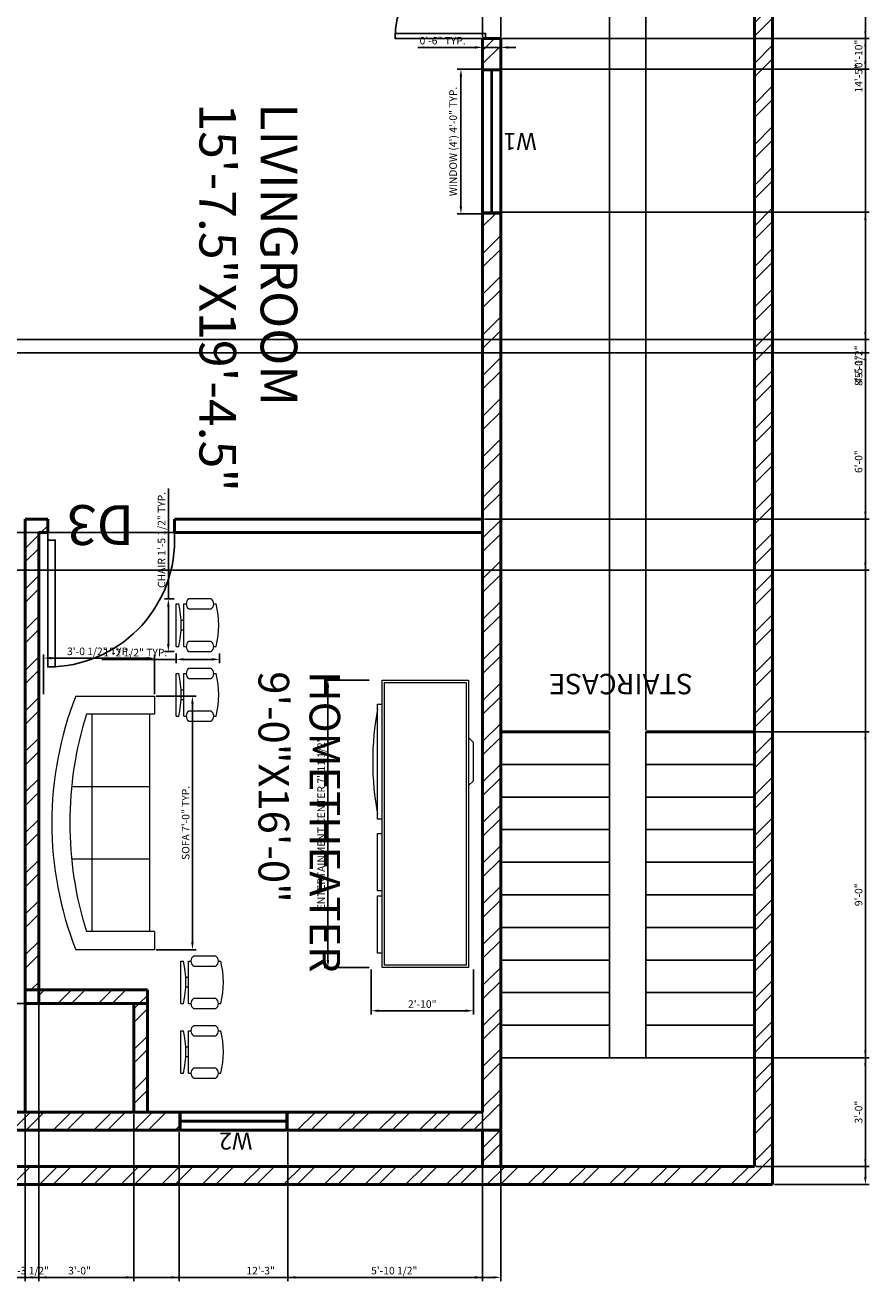
# Model space of a CAD drawing. Units: inches. Extents: x 244 to 2800, y 1060 to 1700.
# Tile 4 of 13: x 1088 to 1368, y 1060 to 1477. Entities that reach past the tile are written whole.
import ezdxf

# ---------------------------------------------------------------- set-up
doc = ezdxf.new("R2010")
doc.units = ezdxf.units.IN
for name, color, linetype, lineweight in [('A-ANNO-DIMS', 2, 'Continuous', 18), ('A-ANNO-TEXT', 1, 'Continuous', 18), ('A-DOOR', 5, 'Continuous', 25), ('A-FLOR-STRS', 6, 'Continuous', 25), ('A-FURN', 9, 'Continuous', 18), ('A-GLAZ', 3, 'Continuous', 25), ('A-WALL', 7, 'Continuous', 50), ('A-WALL-PATT', 8, 'Continuous', 13)]:
    doc.layers.add(name, color=color, linetype=linetype, lineweight=lineweight)
doc.styles.get("Standard").update_dxf_attribs({"font": 'arial.ttf'})
doc.dimstyles.new('ISO-25', dxfattribs={"dimtxt": 2.5, "dimasz": 2.5, "dimexe": 1.25, "dimexo": 0.625, "dimtad": 1, "dimlunit": 4, "dimtxsty": 'Standard', "dimcen": 2.5, "dimadec": 0, "dimazin": 0, "dimtfac": 1, "dimtmove": 0, "dimatfit": 3, "dimfxl": 1, "dimarcsym": 0})

# ---------------------------------------------------------------- blocks, each defined once
blk = doc.blocks.new('*U2')
for p, q in [((0, 0), (0, -5)), ((30, 0), (30, -5))]:
    blk.add_line(p, q)
blk.add_lwpolyline([(0, 0), (0, 30), (1.75, 30), (1.75, 0)], close=True)
blk.add_arc((0, 0), 30, 0, 90)
blk = doc.blocks.new('Entertainment Center')
for p, q in [((-4, 0), (-5, -1)), ((4, 0), (-4, 0)), ((5, -1), (4, 0)), ((-17, -19), (-17, -1)), ((-17, -1), (43, -1)), ((-16.5, -18.5), (-16.5, -1.5)), ((-16.5, -1.5), (42.5, -1.5)), ((42.5, -1.5), (42.5, -18.5)), ((43, -1), (43, -19)), ((43, -19), (-17, -19)), ((42.5, -18.5), (-16.5, -18.5)), ((-12, -20), (-12, -19)), ((12, -20), (-12, -20)), ((12, -19), (12, -20)), ((15, -20), (15, -19)), ((27, -20), (15, -20)), ((27, -19), (27, -20)), ((28, -20), (28, -19)), ((40, -20), (28, -20)), ((40, -19), (40, -20))]:
    blk.add_line(p, q)
blk.add_arc((0, 40), 61, 259.6111, 280.3889)
blk = doc.blocks.new('Chair - Desk')
for p, q in [((-8.5, 0), (-8.5, -1)), ((-8.5, 0), (8.5, 0)), ((8.5, 0), (8.5, -1)), ((-10.5, -5), (-10.5, -14)), ((-8.5, -3), (-8.5, -4)), ((-8.5, -3), (8.5, -3)), ((-6.5, -14), (-6.5, -5)), ((-2, -3), (-2, -1.9355)), ((2, -1.9576), (2, -3)), ((6.5, -5), (6.5, -14)), ((8.5, -3), (8.5, -4)), ((10.5, -14), (10.5, -5)), ((-8.5, -15), (-8.5, -16)), ((8.5, -15), (8.5, -16))]:
    blk.add_line(p, q)
for centre, radius, start, end in [((-8.5, -6.5), 2.5, 36.8699, 143.1301), ((0, 34.625), 36.625, 256.5803, 283.4197), ((8.5, -6.5), 2.5, 36.8699, 143.1301), ((-8.5, -12.5), 2.5, 216.8699, 323.1301), ((8.5, -12.5), 2.5, 216.8699, 323.1301), ((0, 19.625), 36.625, 256.5803, 283.4197)]:
    blk.add_arc(centre, radius, start, end)
blk = doc.blocks.new('Sofa - Roundback 7 ft.')
for p, q in [((-12.00002, -32.4421), (-12.00003, -6.5971)), ((11.99997, -32.4421), (11.99998, -6.5971)), ((-36.000027, -34), (-36.000027, -11.4696)), ((35.99998, -34), (35.99998, -11.4696)), ((-35.999844, -13.3819), (35.9998, -13.3819)), ((-36.000027, -32.4421), (35.99998, -32.4421))]:
    blk.add_line(p, q)
for points in [[(-36.000027, -34), (-42.000027, -34), (-42.000027, -8)], [(41.99998, -8), (41.99998, -34), (35.99998, -34)]]:
    blk.add_lwpolyline(points)
for centre, radius, start, end in [((0, -114.25), 114.25, 68.43141, 111.5686), ((-0.00001, -127.1968), 121.1968, 72.72033, 107.2797)]:
    blk.add_arc(centre, radius, start, end)
blk = doc.blocks.new('WIN-48')
for p, q in [((0, 0), (0, 47.95)), ((0, 47.95), (6, 47.95)), ((6, 47.95), (6, 0)), ((6, 0), (0, 0))]:
    blk.add_line(p, q)
blk = doc.blocks.new('*D52')
at = {"layer": 'A-ANNO-DIMS', "color": 0, "lineweight": -2, "transparency": 16777216}
for p, q in [((1135.65, 1286.99), (1135.65, 1323.61)), ((1137.63, 1286.99), (1134.4, 1286.99)), ((1135.65, 1272.1), (1135.65, 1284.49)), ((1137.63, 1269.6), (1134.4, 1269.6))]:
    blk.add_line(p, q, dxfattribs=at)
at = {"layer": 'A-ANNO-DIMS', "color": 0, "transparency": 16777216}
for points in [[(1135.23, 1284.49), (1136.07, 1284.49), (1135.65, 1286.99)], [(1135.23, 1272.1), (1136.07, 1272.1), (1135.65, 1269.6)]]:
    blk.add_solid(points, dxfattribs=at)
at = {"layer": 'Defpoints', "color": 0, "transparency": 16777216}
for p in [(1135.65, 1286.99), (1138.26, 1286.99), (1138.26, 1269.6)]:
    blk.add_point(p, dxfattribs=at)
at = {"layer": 'A-ANNO-DIMS', "color": 0, "transparency": 16777216, "insert": (1133.73, 1306.55), "char_height": 2.5, "attachment_point": 5, "rotation": 90}
blk.add_mtext('CHAIR 1\'-5 1/2" TYP.', dxfattribs=at)
blk = doc.blocks.new('*D53')
at = {"layer": 'A-ANNO-DIMS', "color": 0, "lineweight": -2, "transparency": 16777216}
for p, q in [((1138.26, 1266.99), (1113.68, 1266.99)), ((1138.26, 1268.98), (1138.26, 1265.74)), ((1150.11, 1266.99), (1140.76, 1266.99)), ((1152.61, 1268.98), (1152.61, 1265.74))]:
    blk.add_line(p, q, dxfattribs=at)
at = {"layer": 'A-ANNO-DIMS', "color": 0, "transparency": 16777216}
for points in [[(1140.76, 1267.41), (1140.76, 1266.58), (1138.26, 1266.99)], [(1150.11, 1267.41), (1150.11, 1266.58), (1152.61, 1266.99)]]:
    blk.add_solid(points, dxfattribs=at)
at = {"layer": 'Defpoints', "color": 0, "transparency": 16777216}
for p in [(1138.26, 1269.6), (1138.26, 1266.99), (1152.61, 1269.6)]:
    blk.add_point(p, dxfattribs=at)
at = {"layer": 'A-ANNO-DIMS', "color": 0, "transparency": 16777216, "insert": (1124.72, 1268.91), "char_height": 2.5, "attachment_point": 5}
blk.add_mtext('1\'-2 1/2" TYP.', dxfattribs=at)
blk = doc.blocks.new('*D58')
at = {"layer": 'A-ANNO-DIMS', "color": 0, "lineweight": -2, "transparency": 16777216}
for p, q in [((1239.11, 1462.54), (1231.29, 1462.54)), ((1232.54, 1460.04), (1232.54, 1417.1)), ((1239.11, 1414.6), (1231.29, 1414.6))]:
    blk.add_line(p, q, dxfattribs=at)
at = {"layer": 'A-ANNO-DIMS', "color": 0, "transparency": 16777216}
for points in [[(1232.13, 1460.04), (1232.96, 1460.04), (1232.54, 1462.54)], [(1232.13, 1417.1), (1232.96, 1417.1), (1232.54, 1414.6)]]:
    blk.add_solid(points, dxfattribs=at)
at = {"layer": 'Defpoints', "color": 0, "transparency": 16777216}
for p in [(1239.74, 1462.54), (1232.54, 1414.6), (1239.74, 1414.6)]:
    blk.add_point(p, dxfattribs=at)
at = {"layer": 'A-ANNO-DIMS', "color": 0, "transparency": 16777216, "insert": (1230.28, 1438.57), "char_height": 2.5, "attachment_point": 5, "rotation": 90}
blk.add_mtext('WINDOW (4\') 4\'-0" TYP.', dxfattribs=at)
blk = doc.blocks.new('*D59')
at = {"layer": 'A-ANNO-DIMS', "color": 0, "lineweight": -2, "transparency": 16777216}
for p, q in [((1239.74, 1463.17), (1239.74, 1470.98)), ((1245.74, 1463.17), (1245.74, 1470.98)), ((1237.24, 1469.73), (1218.25, 1469.73)), ((1245.74, 1469.73), (1239.74, 1469.73)), ((1248.24, 1469.73), (1250.74, 1469.73))]:
    blk.add_line(p, q, dxfattribs=at)
at = {"layer": 'A-ANNO-DIMS', "color": 0, "transparency": 16777216}
for points in [[(1237.24, 1470.15), (1237.24, 1469.32), (1239.74, 1469.73)], [(1248.24, 1470.15), (1248.24, 1469.32), (1245.74, 1469.73)]]:
    blk.add_solid(points, dxfattribs=at)
at = {"layer": 'Defpoints', "color": 0, "transparency": 16777216}
for p in [(1239.74, 1469.73), (1239.74, 1462.54), (1245.74, 1462.54)]:
    blk.add_point(p, dxfattribs=at)
at = {"layer": 'A-ANNO-DIMS', "color": 0, "transparency": 16777216, "insert": (1226.49, 1471.64), "char_height": 2.5, "attachment_point": 5}
blk.add_mtext('0\'-6" TYP.', dxfattribs=at)
blk = doc.blocks.new('*D66')
at = {"layer": 'A-ANNO-DIMS', "color": 0, "lineweight": -2, "transparency": 16777216}
for p, q in [((1131.65, 1254.8), (1144.88, 1254.8)), ((1143.63, 1173.3), (1143.63, 1252.3)), ((1131.65, 1170.8), (1144.88, 1170.8))]:
    blk.add_line(p, q, dxfattribs=at)
at = {"layer": 'A-ANNO-DIMS', "color": 0, "transparency": 16777216}
for points in [[(1143.21, 1252.3), (1144.05, 1252.3), (1143.63, 1254.8)], [(1143.21, 1173.3), (1144.05, 1173.3), (1143.63, 1170.8)]]:
    blk.add_solid(points, dxfattribs=at)
at = {"layer": 'Defpoints', "color": 0, "transparency": 16777216}
for p in [(1131.03, 1254.8), (1143.63, 1254.8), (1131.03, 1170.8)]:
    blk.add_point(p, dxfattribs=at)
at = {"layer": 'A-ANNO-DIMS', "color": 0, "transparency": 16777216, "insert": (1141.71, 1212.8), "char_height": 2.5, "attachment_point": 5, "rotation": 90}
blk.add_mtext('SOFA 7\'-0" TYP.', dxfattribs=at)
blk = doc.blocks.new('*D67')
at = {"layer": 'A-ANNO-DIMS', "color": 0, "lineweight": -2, "transparency": 16777216}
for p, q in [((1094.36, 1255.42), (1094.36, 1268.65)), ((1128.53, 1267.4), (1096.86, 1267.4)), ((1131.03, 1255.42), (1131.03, 1268.65))]:
    blk.add_line(p, q, dxfattribs=at)
at = {"layer": 'A-ANNO-DIMS', "color": 0, "transparency": 16777216}
for points in [[(1096.86, 1267.82), (1096.86, 1266.98), (1094.36, 1267.4)], [(1128.53, 1267.82), (1128.53, 1266.98), (1131.03, 1267.4)]]:
    blk.add_solid(points, dxfattribs=at)
at = {"layer": 'Defpoints', "color": 0, "transparency": 16777216}
for p in [(1094.36, 1267.4), (1094.36, 1254.8), (1131.03, 1254.8)]:
    blk.add_point(p, dxfattribs=at)
at = {"layer": 'A-ANNO-DIMS', "color": 0, "transparency": 16777216, "insert": (1112.7, 1269.32), "char_height": 2.5, "attachment_point": 5}
blk.add_mtext('3\'-0 1/2" TYP.', dxfattribs=at)
blk = doc.blocks.new('*D68')
at = {"layer": 'A-ANNO-DIMS', "color": 0, "lineweight": -2, "transparency": 16777216}
for p, q in [((1202.17, 1260.11), (1187.26, 1260.11)), ((1188.51, 1257.61), (1188.51, 1167.36)), ((1202.17, 1164.86), (1187.26, 1164.86))]:
    blk.add_line(p, q, dxfattribs=at)
at = {"layer": 'A-ANNO-DIMS', "color": 0, "transparency": 16777216}
for points in [[(1188.09, 1257.61), (1188.92, 1257.61), (1188.51, 1260.11)], [(1188.09, 1167.36), (1188.92, 1167.36), (1188.51, 1164.86)]]:
    blk.add_solid(points, dxfattribs=at)
at = {"layer": 'Defpoints', "color": 0, "transparency": 16777216}
for p in [(1202.79, 1260.11), (1188.51, 1164.86), (1202.79, 1164.86)]:
    blk.add_point(p, dxfattribs=at)
at = {"layer": 'A-ANNO-DIMS', "color": 0, "transparency": 16777216, "insert": (1186.59, 1212.49), "char_height": 2.5, "attachment_point": 5, "rotation": 90}
blk.add_mtext('ENTERTAINMENT CENTER 7\'-11 1/2"', dxfattribs=at)
blk = doc.blocks.new('*D69')
at = {"layer": 'A-ANNO-DIMS', "color": 0, "lineweight": -2, "transparency": 16777216}
for p, q in [((1202.79, 1164.24), (1202.79, 1149.32)), ((1236.66, 1164.24), (1236.66, 1149.32)), ((1205.29, 1150.57), (1234.16, 1150.57))]:
    blk.add_line(p, q, dxfattribs=at)
at = {"layer": 'A-ANNO-DIMS', "color": 0, "transparency": 16777216}
for points in [[(1205.29, 1150.99), (1205.29, 1150.16), (1202.79, 1150.57)], [(1234.16, 1150.99), (1234.16, 1150.16), (1236.66, 1150.57)]]:
    blk.add_solid(points, dxfattribs=at)
at = {"layer": 'Defpoints', "color": 0, "transparency": 16777216}
for p in [(1202.79, 1164.86), (1236.66, 1164.86), (1236.66, 1150.57)]:
    blk.add_point(p, dxfattribs=at)
at = {"layer": 'A-ANNO-DIMS', "color": 0, "transparency": 16777216, "insert": (1219.73, 1152.47), "char_height": 2.5, "attachment_point": 5}
blk.add_mtext('2\'-10"', dxfattribs=at)
blk = doc.blocks.new('*D108')
at = {"layer": 'A-ANNO-DIMS', "color": 0, "lineweight": -2, "transparency": 16777216}
for p, q in [((1336.36, 1632.99), (1367.74, 1632.99)), ((1366.49, 1095.49), (1366.49, 1630.49)), ((1336.36, 1092.99), (1367.74, 1092.99))]:
    blk.add_line(p, q, dxfattribs=at)
at = {"layer": 'A-ANNO-DIMS', "color": 0, "transparency": 16777216}
for points in [[(1366.07, 1630.49), (1366.9, 1630.49), (1366.49, 1632.99)], [(1366.07, 1095.49), (1366.9, 1095.49), (1366.49, 1092.99)]]:
    blk.add_solid(points, dxfattribs=at)
at = {"layer": 'Defpoints', "color": 0, "transparency": 16777216}
for p in [(1335.74, 1632.99), (1366.49, 1632.99), (1335.74, 1092.99)]:
    blk.add_point(p, dxfattribs=at)
at = {"layer": 'A-ANNO-DIMS', "color": 0, "transparency": 16777216, "insert": (1364.58, 1362.99), "char_height": 2.5, "attachment_point": 5, "rotation": 90}
blk.add_mtext('45\'-0"', dxfattribs=at)
blk = doc.blocks.new('*D124')
at = {"layer": 'A-ANNO-DIMS', "color": 0, "lineweight": -2, "transparency": 16777216}
for p, q in [((962.86, 1368.49), (1367.74, 1368.49)), ((1366.49, 1298.99), (1366.49, 1365.99)), ((962.86, 1296.49), (1367.74, 1296.49))]:
    blk.add_line(p, q, dxfattribs=at)
at = {"layer": 'A-ANNO-DIMS', "color": 0, "transparency": 16777216}
for points in [[(1366.07, 1365.99), (1366.9, 1365.99), (1366.49, 1368.49)], [(1366.07, 1298.99), (1366.9, 1298.99), (1366.49, 1296.49)]]:
    blk.add_solid(points, dxfattribs=at)
at = {"layer": 'Defpoints', "color": 0, "transparency": 16777216}
for p in [(962.24, 1368.49), (1366.49, 1368.49), (962.24, 1296.49)]:
    blk.add_point(p, dxfattribs=at)
at = {"layer": 'A-ANNO-DIMS', "color": 0, "transparency": 16777216, "insert": (1364.58, 1332.49), "char_height": 2.5, "attachment_point": 5, "rotation": 90}
blk.add_mtext('6\'-0"', dxfattribs=at)
blk = doc.blocks.new('*D125')
at = {"layer": 'A-ANNO-DIMS', "color": 0, "lineweight": -2, "transparency": 16777216}
for p, q in [((880.36, 1545.99), (1367.74, 1545.99)), ((1366.49, 1375.49), (1366.49, 1543.49)), ((880.36, 1372.99), (1367.74, 1372.99))]:
    blk.add_line(p, q, dxfattribs=at)
at = {"layer": 'A-ANNO-DIMS', "color": 0, "transparency": 16777216}
for points in [[(1366.07, 1543.49), (1366.9, 1543.49), (1366.49, 1545.99)], [(1366.07, 1375.49), (1366.9, 1375.49), (1366.49, 1372.99)]]:
    blk.add_solid(points, dxfattribs=at)
at = {"layer": 'Defpoints', "color": 0, "transparency": 16777216}
for p in [(879.74, 1545.99), (1366.49, 1545.99), (879.74, 1372.99)]:
    blk.add_point(p, dxfattribs=at)
at = {"layer": 'A-ANNO-DIMS', "color": 0, "transparency": 16777216, "insert": (1364.58, 1459.49), "char_height": 2.5, "attachment_point": 5, "rotation": 90}
blk.add_mtext('14\'-5"', dxfattribs=at)
blk = doc.blocks.new('*D129')
at = {"layer": 'A-ANNO-DIMS', "color": 0, "lineweight": -2, "transparency": 16777216}
for p, q in [((1039.6, 1110.36), (1039.6, 1060.99)), ((1139.24, 1110.36), (1139.24, 1060.99)), ((1042.1, 1062.24), (1136.74, 1062.24))]:
    blk.add_line(p, q, dxfattribs=at)
at = {"layer": 'A-ANNO-DIMS', "color": 0, "transparency": 16777216}
for points in [[(1042.1, 1062.65), (1042.1, 1061.82), (1039.6, 1062.24)], [(1136.74, 1062.65), (1136.74, 1061.82), (1139.24, 1062.24)]]:
    blk.add_solid(points, dxfattribs=at)
at = {"layer": 'Defpoints', "color": 0, "transparency": 16777216}
for p in [(1039.6, 1110.99), (1139.24, 1110.99), (1139.24, 1062.24)]:
    blk.add_point(p, dxfattribs=at)
at = {"layer": 'A-ANNO-DIMS', "color": 0, "transparency": 16777216, "insert": (1089.42, 1064.15), "char_height": 2.5, "attachment_point": 5}
blk.add_mtext('8\'-3 1/2"', dxfattribs=at)
blk = doc.blocks.new('*D130')
at = {"layer": 'A-ANNO-DIMS', "color": 0, "lineweight": -2, "transparency": 16777216}
for p, q in [((1175.18, 1110.36), (1175.18, 1060.99)), ((1245.74, 1110.36), (1245.74, 1060.99)), ((1177.68, 1062.24), (1243.24, 1062.24))]:
    blk.add_line(p, q, dxfattribs=at)
at = {"layer": 'A-ANNO-DIMS', "color": 0, "transparency": 16777216}
for points in [[(1177.68, 1062.65), (1177.68, 1061.82), (1175.18, 1062.24)], [(1243.24, 1062.65), (1243.24, 1061.82), (1245.74, 1062.24)]]:
    blk.add_solid(points, dxfattribs=at)
at = {"layer": 'Defpoints', "color": 0, "transparency": 16777216}
for p in [(1175.18, 1110.99), (1245.74, 1110.99), (1245.74, 1062.24)]:
    blk.add_point(p, dxfattribs=at)
at = {"layer": 'A-ANNO-DIMS', "color": 0, "transparency": 16777216, "insert": (1210.46, 1064.15), "char_height": 2.5, "attachment_point": 5}
blk.add_mtext('5\'-10 1/2"', dxfattribs=at)
blk = doc.blocks.new('*D132')
at = {"layer": 'A-ANNO-DIMS', "color": 0, "lineweight": -2, "transparency": 16777216}
for p, q in [((1088.24, 1116.36), (1088.24, 1060.99)), ((1124.24, 1116.36), (1124.24, 1060.99)), ((1090.74, 1062.24), (1121.74, 1062.24))]:
    blk.add_line(p, q, dxfattribs=at)
at = {"layer": 'A-ANNO-DIMS', "color": 0, "transparency": 16777216}
for points in [[(1090.74, 1062.65), (1090.74, 1061.82), (1088.24, 1062.24)], [(1121.74, 1062.65), (1121.74, 1061.82), (1124.24, 1062.24)]]:
    blk.add_solid(points, dxfattribs=at)
at = {"layer": 'Defpoints', "color": 0, "transparency": 16777216}
for p in [(1088.24, 1116.99), (1124.24, 1116.99), (1124.24, 1062.24)]:
    blk.add_point(p, dxfattribs=at)
at = {"layer": 'A-ANNO-DIMS', "color": 0, "transparency": 16777216, "insert": (1106.24, 1064.14), "char_height": 2.5, "attachment_point": 5}
blk.add_mtext('3\'-0"', dxfattribs=at)
blk = doc.blocks.new('*D133')
at = {"layer": 'A-ANNO-DIMS', "color": 0, "lineweight": -2, "transparency": 16777216}
for p, q in [((1123.61, 1152.99), (823.74, 1152.99)), ((824.99, 1119.49), (824.99, 1150.49)), ((1123.61, 1116.99), (823.74, 1116.99))]:
    blk.add_line(p, q, dxfattribs=at)
at = {"layer": 'A-ANNO-DIMS', "color": 0, "transparency": 16777216}
for points in [[(824.57, 1150.49), (825.4, 1150.49), (824.99, 1152.99)], [(824.57, 1119.49), (825.4, 1119.49), (824.99, 1116.99)]]:
    blk.add_solid(points, dxfattribs=at)
at = {"layer": 'Defpoints', "color": 0, "transparency": 16777216}
for p in [(824.99, 1152.99), (1124.24, 1152.99), (1124.24, 1116.99)]:
    blk.add_point(p, dxfattribs=at)
at = {"layer": 'A-ANNO-DIMS', "color": 0, "transparency": 16777216, "insert": (823.08, 1134.99), "char_height": 2.5, "attachment_point": 5, "rotation": 90}
blk.add_mtext('3\'-0"', dxfattribs=at)
blk = doc.blocks.new('*D134')
at = {"layer": 'A-ANNO-DIMS', "color": 0, "lineweight": -2, "transparency": 16777216}
for p, q in [((1239.11, 1308.99), (823.74, 1308.99)), ((824.99, 1119.49), (824.99, 1306.49)), ((1239.11, 1116.99), (823.74, 1116.99))]:
    blk.add_line(p, q, dxfattribs=at)
at = {"layer": 'A-ANNO-DIMS', "color": 0, "transparency": 16777216}
for points in [[(824.57, 1306.49), (825.4, 1306.49), (824.99, 1308.99)], [(824.57, 1119.49), (825.4, 1119.49), (824.99, 1116.99)]]:
    blk.add_solid(points, dxfattribs=at)
at = {"layer": 'Defpoints', "color": 0, "transparency": 16777216}
for p in [(824.99, 1308.99), (1239.74, 1308.99), (1239.74, 1116.99)]:
    blk.add_point(p, dxfattribs=at)
at = {"layer": 'A-ANNO-DIMS', "color": 0, "transparency": 16777216, "insert": (823.08, 1212.99), "char_height": 2.5, "attachment_point": 5, "rotation": 90}
blk.add_mtext('16\'-0"', dxfattribs=at)
blk = doc.blocks.new('*D135')
at = {"layer": 'A-ANNO-DIMS', "color": 0, "lineweight": -2, "transparency": 16777216}
for p, q in [((1092.74, 1308.36), (1092.74, 1060.99)), ((1239.74, 1308.36), (1239.74, 1060.99)), ((1095.24, 1062.24), (1237.24, 1062.24))]:
    blk.add_line(p, q, dxfattribs=at)
at = {"layer": 'A-ANNO-DIMS', "color": 0, "transparency": 16777216}
for points in [[(1095.24, 1062.65), (1095.24, 1061.82), (1092.74, 1062.24)], [(1237.24, 1062.65), (1237.24, 1061.82), (1239.74, 1062.24)]]:
    blk.add_solid(points, dxfattribs=at)
at = {"layer": 'Defpoints', "color": 0, "transparency": 16777216}
for p in [(1092.74, 1308.99), (1239.74, 1308.99), (1239.74, 1062.24)]:
    blk.add_point(p, dxfattribs=at)
at = {"layer": 'A-ANNO-DIMS', "color": 0, "transparency": 16777216, "insert": (1166.24, 1064.14), "char_height": 2.5, "attachment_point": 5}
blk.add_mtext('12\'-3"', dxfattribs=at)
blk = doc.blocks.new('*D139')
at = {"layer": 'A-ANNO-DIMS', "color": 0, "lineweight": -2, "transparency": 16777216}
for p, q in [((1246.36, 1415.1), (1367.74, 1415.1)), ((1366.49, 1315.99), (1366.49, 1412.6)), ((1240.36, 1313.49), (1367.74, 1313.49))]:
    blk.add_line(p, q, dxfattribs=at)
at = {"layer": 'A-ANNO-DIMS', "color": 0, "transparency": 16777216}
for points in [[(1366.07, 1412.6), (1366.9, 1412.6), (1366.49, 1415.1)], [(1366.07, 1315.99), (1366.9, 1315.99), (1366.49, 1313.49)]]:
    blk.add_solid(points, dxfattribs=at)
at = {"layer": 'Defpoints', "color": 0, "transparency": 16777216}
for p in [(1245.74, 1415.1), (1366.49, 1415.1), (1239.74, 1313.49)]:
    blk.add_point(p, dxfattribs=at)
at = {"layer": 'A-ANNO-DIMS', "color": 0, "transparency": 16777216, "insert": (1364.57, 1364.29), "char_height": 2.5, "attachment_point": 5, "rotation": 90}
blk.add_mtext('8\'-5 1/2"', dxfattribs=at)
blk = doc.blocks.new('*D140')
at = {"layer": 'A-ANNO-DIMS', "color": 0, "lineweight": -2, "transparency": 16777216}
for p, q in [((1246.36, 1472.64), (1367.74, 1472.64)), ((1366.49, 1465.04), (1366.49, 1470.14)), ((1246.36, 1462.54), (1367.74, 1462.54))]:
    blk.add_line(p, q, dxfattribs=at)
at = {"layer": 'A-ANNO-DIMS', "color": 0, "transparency": 16777216}
for points in [[(1366.07, 1470.14), (1366.9, 1470.14), (1366.49, 1472.64)], [(1366.07, 1465.04), (1366.9, 1465.04), (1366.49, 1462.54)]]:
    blk.add_solid(points, dxfattribs=at)
at = {"layer": 'Defpoints', "color": 0, "transparency": 16777216}
for p in [(1245.74, 1472.64), (1366.49, 1472.64), (1245.74, 1462.54)]:
    blk.add_point(p, dxfattribs=at)
at = {"layer": 'A-ANNO-DIMS', "color": 0, "transparency": 16777216, "insert": (1364.58, 1467.59), "char_height": 2.5, "attachment_point": 5, "rotation": 90}
blk.add_mtext('0\'-10"', dxfattribs=at)
blk = doc.blocks.new('*D141')
at = {"layer": 'A-ANNO-DIMS', "color": 0, "lineweight": -2, "transparency": 16777216}
for p, q in [((1246.36, 1532.64), (1367.74, 1532.64)), ((1366.49, 1475.14), (1366.49, 1530.14)), ((1246.36, 1472.64), (1367.74, 1472.64))]:
    blk.add_line(p, q, dxfattribs=at)
at = {"layer": 'A-ANNO-DIMS', "color": 0, "transparency": 16777216}
for points in [[(1366.07, 1530.14), (1366.9, 1530.14), (1366.49, 1532.64)], [(1366.07, 1475.14), (1366.9, 1475.14), (1366.49, 1472.64)]]:
    blk.add_solid(points, dxfattribs=at)
at = {"layer": 'Defpoints', "color": 0, "transparency": 16777216}
for p in [(1245.74, 1532.64), (1366.49, 1532.64), (1245.74, 1472.64)]:
    blk.add_point(p, dxfattribs=at)
at = {"layer": 'A-ANNO-DIMS', "color": 0, "transparency": 16777216, "insert": (1364.58, 1502.64), "char_height": 2.5, "attachment_point": 5, "rotation": 90}
blk.add_mtext('5\'-0"', dxfattribs=at)
blk = doc.blocks.new('*D143')
at = {"layer": 'A-ANNO-DIMS', "color": 0, "lineweight": -2, "transparency": 16777216}
for p, q in [((1330.36, 1134.99), (1367.74, 1134.99)), ((1366.49, 1101.49), (1366.49, 1132.49)), ((1330.36, 1098.99), (1367.74, 1098.99))]:
    blk.add_line(p, q, dxfattribs=at)
at = {"layer": 'A-ANNO-DIMS', "color": 0, "transparency": 16777216}
for points in [[(1366.07, 1132.49), (1366.9, 1132.49), (1366.49, 1134.99)], [(1366.07, 1101.49), (1366.9, 1101.49), (1366.49, 1098.99)]]:
    blk.add_solid(points, dxfattribs=at)
at = {"layer": 'Defpoints', "color": 0, "transparency": 16777216}
for p in [(1329.74, 1134.99), (1366.49, 1134.99), (1329.74, 1098.99)]:
    blk.add_point(p, dxfattribs=at)
at = {"layer": 'A-ANNO-DIMS', "color": 0, "transparency": 16777216, "insert": (1364.58, 1116.99), "char_height": 2.5, "attachment_point": 5, "rotation": 90}
blk.add_mtext('3\'-0"', dxfattribs=at)
blk = doc.blocks.new('*D144')
at = {"layer": 'A-ANNO-DIMS', "color": 0, "lineweight": -2, "transparency": 16777216}
for p, q in [((1330.36, 1242.99), (1367.74, 1242.99)), ((1366.49, 1137.49), (1366.49, 1240.49)), ((1330.36, 1134.99), (1367.74, 1134.99))]:
    blk.add_line(p, q, dxfattribs=at)
at = {"layer": 'A-ANNO-DIMS', "color": 0, "transparency": 16777216}
for points in [[(1366.07, 1240.49), (1366.9, 1240.49), (1366.49, 1242.99)], [(1366.07, 1137.49), (1366.9, 1137.49), (1366.49, 1134.99)]]:
    blk.add_solid(points, dxfattribs=at)
at = {"layer": 'Defpoints', "color": 0, "transparency": 16777216}
for p in [(1329.74, 1242.99), (1366.49, 1242.99), (1329.74, 1134.99)]:
    blk.add_point(p, dxfattribs=at)
at = {"layer": 'A-ANNO-DIMS', "color": 0, "transparency": 16777216, "insert": (1364.58, 1188.99), "char_height": 2.5, "attachment_point": 5, "rotation": 90}
blk.add_mtext('9\'-0"', dxfattribs=at)
blk = doc.blocks.new('*D145')
at = {"layer": 'A-ANNO-DIMS', "color": 0, "lineweight": -2, "transparency": 16777216}
for p, q in [((1245.74, 1243.61), (1245.74, 1664.99)), ((1248.24, 1663.74), (1279.24, 1663.74)), ((1281.74, 1243.61), (1281.74, 1664.99))]:
    blk.add_line(p, q, dxfattribs=at)
at = {"layer": 'A-ANNO-DIMS', "color": 0, "transparency": 16777216}
for points in [[(1248.24, 1664.15), (1248.24, 1663.32), (1245.74, 1663.74)], [(1279.24, 1664.15), (1279.24, 1663.32), (1281.74, 1663.74)]]:
    blk.add_solid(points, dxfattribs=at)
at = {"layer": 'Defpoints', "color": 0, "transparency": 16777216}
for p in [(1281.74, 1663.74), (1245.74, 1242.99), (1281.74, 1242.99)]:
    blk.add_point(p, dxfattribs=at)
at = {"layer": 'A-ANNO-DIMS', "color": 0, "transparency": 16777216, "insert": (1263.74, 1665.64), "char_height": 2.5, "attachment_point": 5}
blk.add_mtext('3\'-0"', dxfattribs=at)
blk = doc.blocks.new('*D146')
at = {"layer": 'A-ANNO-DIMS', "color": 0, "lineweight": -2, "transparency": 16777216}
for p, q in [((1293.74, 1243.61), (1293.74, 1664.99)), ((1296.24, 1663.74), (1327.24, 1663.74)), ((1329.74, 1243.61), (1329.74, 1664.99))]:
    blk.add_line(p, q, dxfattribs=at)
at = {"layer": 'A-ANNO-DIMS', "color": 0, "transparency": 16777216}
for points in [[(1296.24, 1664.15), (1296.24, 1663.32), (1293.74, 1663.74)], [(1327.24, 1664.15), (1327.24, 1663.32), (1329.74, 1663.74)]]:
    blk.add_solid(points, dxfattribs=at)
at = {"layer": 'Defpoints', "color": 0, "transparency": 16777216}
for p in [(1329.74, 1663.74), (1293.74, 1242.99), (1329.74, 1242.99)]:
    blk.add_point(p, dxfattribs=at)
at = {"layer": 'A-ANNO-DIMS', "color": 0, "transparency": 16777216, "insert": (1311.74, 1665.64), "char_height": 2.5, "attachment_point": 5}
blk.add_mtext('3\'-0"', dxfattribs=at)
blk = doc.blocks.new('*D147')
at = {"layer": 'A-ANNO-DIMS', "color": 0, "lineweight": -2, "transparency": 16777216}
for p, q in [((1052.24, 1491.26), (1052.24, 1664.99)), ((1054.74, 1663.74), (1237.24, 1663.74)), ((1239.74, 1473.26), (1239.74, 1664.99))]:
    blk.add_line(p, q, dxfattribs=at)
at = {"layer": 'A-ANNO-DIMS', "color": 0, "transparency": 16777216}
for points in [[(1054.74, 1664.15), (1054.74, 1663.32), (1052.24, 1663.74)], [(1237.24, 1664.15), (1237.24, 1663.32), (1239.74, 1663.74)]]:
    blk.add_solid(points, dxfattribs=at)
at = {"layer": 'Defpoints', "color": 0, "transparency": 16777216}
for p in [(1239.74, 1663.74), (1052.24, 1490.64), (1239.74, 1472.64)]:
    blk.add_point(p, dxfattribs=at)
at = {"layer": 'A-ANNO-DIMS', "color": 0, "transparency": 16777216, "insert": (1145.99, 1665.65), "char_height": 2.5, "attachment_point": 5}
blk.add_mtext('15\'-7 1/2"', dxfattribs=at)

msp = doc.modelspace()

# ---------------------------------------------------------------- hatches: boundary and pattern name
at = {"layer": 'A-WALL-PATT'}
h = msp.add_hatch(dxfattribs=at)
h.set_pattern_fill('ANSI32', color=256)
h.paths.add_polyline_path([(1335.736, 1632.986), (855.736, 1632.986), (855.736, 1092.986), (1335.736, 1092.986)])
h.paths.add_polyline_path([(1329.736, 1626.986), (1329.736, 1098.986), (1245.736, 1098.986), (861.736, 1098.986), (861.736, 1626.986)], flags=16)
h.paths.add_polyline_path([(1245.736, 1551.986), (1245.736, 1532.64), (1239.736, 1532.64), (1239.736, 1545.986), (1137.736, 1545.986), (1137.736, 1551.986)], flags=0)
h.paths.add_polyline_path([(1196.984, 1551.986), (1196.984, 1545.986), (1161.039, 1545.986), (1161.039, 1551.986)], flags=0)
h.paths.add_polyline_path([(1196.484, 1548.786), (1161.539, 1548.786), (1161.539, 1549.186), (1196.484, 1549.186)], flags=0)
h.paths.add_polyline_path([(1245.736, 1472.64), (1245.736, 1242.986), (1281.736, 1242.986), (1281.736, 1134.986), (1293.736, 1134.986), (1293.736, 1242.986), (1329.736, 1242.986), (1329.736, 1134.986), (1245.736, 1134.986), (1245.736, 1110.986), (1139.236, 1110.986), (873.736, 1110.986), (873.736, 1484.64), (879.736, 1484.64), (879.736, 1372.986), (1014.736, 1372.986), (1014.736, 1368.486), (965.236, 1368.486), (965.236, 1296.486), (1047.736, 1296.486), (1047.736, 1368.486), (1044.736, 1368.486), (1044.736, 1372.986), (1047.736, 1372.986), (1047.736, 1490.64), (1052.236, 1490.64), (1052.236, 1288.986), (1047.736, 1288.986), (1047.736, 1291.986), (912.736, 1291.986), (912.736, 1296.486), (962.236, 1296.486), (962.236, 1368.486), (879.736, 1368.486), (879.736, 1296.486), (882.736, 1296.486), (882.736, 1291.986), (879.736, 1291.986), (879.736, 1116.986), (1047.736, 1116.986), (1047.736, 1246.986), (1052.236, 1246.986), (1052.236, 1116.986), (1088.236, 1116.986), (1088.236, 1152.986), (1088.236, 1313.486), (1095.736, 1313.486), (1095.736, 1308.986), (1092.736, 1308.986), (1092.736, 1157.486), (1128.736, 1157.486), (1128.736, 1116.986), (1139.236, 1116.986), (1175.181, 1116.986), (1239.736, 1116.986), (1239.736, 1308.986), (1137.736, 1308.986), (1137.736, 1313.486), (1239.736, 1313.486), (1239.736, 1472.64)], flags=0)
h.paths.add_polyline_path([(1245.736, 1462.542), (1245.736, 1414.597), (1239.736, 1414.597), (1239.736, 1462.542)], flags=0)
h.paths.add_polyline_path([(1242.936, 1462.042), (1242.936, 1415.097), (1242.536, 1415.097), (1242.536, 1462.042)], flags=0)
h.paths.add_polyline_path([(1095.736, 1551.986), (1095.736, 1545.986), (1052.236, 1545.986), (1052.236, 1532.64), (1047.736, 1532.64), (1047.736, 1545.986), (879.736, 1545.986), (879.736, 1532.64), (873.736, 1532.64), (873.736, 1551.986), (865.04, 1551.986), (865.04, 1623.986), (949.04, 1623.986), (949.04, 1551.986)], flags=0)
h.paths.add_polyline_path([(1020.681, 1551.986), (1020.681, 1545.986), (984.736, 1545.986), (984.736, 1551.986)], flags=0)
h.paths.add_polyline_path([(1020.181, 1548.786), (985.236, 1548.786), (985.236, 1549.186), (1020.181, 1549.186)], flags=0)
h.paths.add_polyline_path([(879.736, 1347.762), (879.736, 1323.817), (873.736, 1323.817), (873.736, 1347.762)], flags=0)
h.paths.add_polyline_path([(876.936, 1347.262), (876.936, 1324.317), (876.536, 1324.317), (876.536, 1347.262)], flags=0)
h.paths.add_polyline_path([(1124.236, 1152.986), (1124.236, 1116.986), (1088.236, 1116.986), (1088.236, 1152.986)], flags=0)
h.paths.add_polyline_path([(879.736, 1287.983), (879.736, 1252.038), (873.736, 1252.038), (873.736, 1287.983)], flags=0)
h.paths.add_polyline_path([(876.936, 1287.483), (876.936, 1252.538), (876.536, 1252.538), (876.536, 1287.483)], flags=0)
h.paths.add_polyline_path([(1175.181, 1116.986), (1175.181, 1110.986), (1139.236, 1110.986), (1139.236, 1114.186), (1174.681, 1114.186), (1174.681, 1116.986)], flags=0)
h.paths.add_polyline_path([(1040.103, 1116.986), (1040.103, 1110.986), (1004.158, 1110.986), (1004.158, 1116.986)], flags=0)
h.paths.add_polyline_path([(1039.603, 1113.786), (1004.658, 1113.786), (1004.658, 1114.186), (1039.603, 1114.186)], flags=0)
h.paths.add_polyline_path([(1164.972, 1113.308), (1150.368, 1113.308), (1150.368, 1101.713), (1164.972, 1101.713)], flags=8)
h.paths.add_polyline_path([(1033.179, 1112.552), (1018.576, 1112.552), (1018.576, 1100.958), (1033.179, 1100.958)], flags=8)
h.paths.add_polyline_path([(874.571, 1270.316), (859.967, 1270.316), (859.967, 1258.722), (874.571, 1258.722)], flags=24)
h.paths.add_polyline_path([(1011.225, 1564.465), (996.622, 1564.465), (996.622, 1552.871), (1011.225, 1552.871)], flags=8)
h.paths.add_polyline_path([(1187.63, 1564.482), (1173.026, 1564.482), (1173.026, 1552.887), (1187.63, 1552.887)], flags=8)
h.paths.add_polyline_path([(1259.132, 1444.47), (1244.529, 1444.47), (1244.529, 1432.875), (1259.132, 1432.875)], flags=8)
h.paths.add_polyline_path([(875.239, 1344.511), (860.635, 1344.511), (860.635, 1332.916), (875.239, 1332.916)], flags=24)
h.paths.add_polyline_path([(892.18, 1510.489), (862.03, 1510.489), (862.03, 1483.307), (892.18, 1483.307)], flags=8)
h.paths.add_polyline_path([(912.199, 1310.068), (882.049, 1310.068), (882.049, 1282.887), (912.199, 1282.887)], flags=8)
h.paths.add_polyline_path([(1043.03, 1389.229), (1012.88, 1389.229), (1012.88, 1362.047), (1043.03, 1362.047)], flags=8)
h.paths.add_polyline_path([(1058.3, 1285.41), (1028.149, 1285.41), (1028.149, 1258.229), (1058.3, 1258.229)], flags=8)
h.paths.add_polyline_path([(1129.051, 1325.331), (1098.901, 1325.331), (1098.901, 1298.15), (1129.051, 1298.15)], flags=8)
h.paths.add_polyline_path([(1063.761, 1526.078), (1033.611, 1526.078), (1033.611, 1498.897), (1063.761, 1498.897)], flags=8)
h.paths.add_polyline_path([(1130.374, 1573.756), (1100.224, 1573.756), (1100.224, 1546.575), (1130.374, 1546.575)], flags=8)
h.paths.add_polyline_path([(1275.672, 1516.103), (1245.522, 1516.103), (1245.522, 1488.922), (1275.672, 1488.922)], flags=8)
h.paths.add_polyline_path([(979.613, 1573.477), (979.613, 1615.869), (957.159, 1615.869), (957.159, 1573.477)], flags=8)
h.paths.add_polyline_path([(1311.481, 1266.003), (1254.484, 1266.003), (1254.484, 1252.05), (1311.481, 1252.05)], flags=8)
h.paths.add_polyline_path([(1159.757, 1266.713), (1159.757, 1153.038), (1197.594, 1153.038), (1197.594, 1266.713)], flags=8)
h.paths.add_polyline_path([(1139.055, 1456.095), (1139.055, 1323.863), (1184.409, 1323.863), (1184.409, 1456.095)], flags=8)
h.paths.add_polyline_path([(936.318, 1364.302), (878.595, 1364.302), (878.595, 1333.511), (936.318, 1333.511)], flags=8)
h.paths.add_polyline_path([(1042.961, 1335.109), (985.238, 1335.109), (985.238, 1304.318), (1042.961, 1304.318)], flags=8)
h.paths.add_polyline_path([(1002.135, 1273.839), (885.452, 1273.839), (885.452, 1222.91), (1002.135, 1222.91)], flags=8)
h.paths.add_polyline_path([(1009.771, 1532.646), (893.088, 1532.646), (893.088, 1481.717), (1009.771, 1481.717)], flags=8)
h = msp.add_hatch(dxfattribs=at)
h.set_pattern_fill('ANSI32', color=256)
h.paths.add_polyline_path([(1245.736, 1472.64), (1240.736, 1472.64), (1239.736, 1472.64), (1239.736, 1462.542), (1245.736, 1462.542)])
h = msp.add_hatch(dxfattribs=at)
h.set_pattern_fill('ANSI32', color=256)
h.paths.add_polyline_path([(1245.736, 1414.597), (1239.736, 1414.597), (1239.736, 1116.986), (1175.181, 1116.986), (1175.181, 1110.986), (1245.736, 1110.986)])
h = msp.add_hatch(dxfattribs=at)
h.set_pattern_fill('ANSI32', color=256)
h.paths.add_polyline_path([(1092.736, 1308.986), (1095.736, 1308.986), (1095.736, 1313.486), (1088.236, 1313.486), (1088.236, 1157.486), (1092.736, 1157.486)])
h = msp.add_hatch(dxfattribs=at)
h.set_pattern_fill('ANSI32', color=256)
h.paths.add_polyline_path([(1128.736, 1157.486), (1092.736, 1157.486), (1092.736, 1152.986), (1128.736, 1152.986)])
h = msp.add_hatch(dxfattribs=at)
h.set_pattern_fill('ANSI32', color=256)
h.paths.add_polyline_path([(1128.736, 1152.986), (1124.236, 1152.986), (1124.236, 1116.986), (1128.736, 1116.986)])
h = msp.add_hatch(dxfattribs=at)
h.set_pattern_fill('ANSI32', color=256)
h.paths.add_polyline_path([(1139.236, 1116.986), (1128.736, 1116.986), (1040.103, 1116.986), (1040.103, 1110.986), (1139.236, 1110.986)])
h = msp.add_hatch(dxfattribs=at)
h.set_pattern_fill('ANSI32', color=256)
h.paths.add_polyline_path([(1245.736, 1110.986), (1239.736, 1110.986), (1239.736, 1098.986), (1245.736, 1098.986)])

# ---------------------------------------------------------------- linework, layer by layer
at = {"layer": 'A-FLOR-STRS'}
for p, q in [((1245.736, 1242.986), (1281.736, 1242.986)), ((1245.736, 1242.986), (1245.736, 1098.986)), ((1245.736, 1242.986), (1281.736, 1242.986)), ((1281.736, 1242.986), (1281.736, 1134.986)), ((1293.736, 1242.986), (1329.736, 1242.986)), ((1293.736, 1242.986), (1293.736, 1134.986)), ((1293.736, 1242.986), (1329.736, 1242.986)), ((1329.736, 1242.986), (1329.736, 1098.986)), ((1245.736, 1232.186), (1281.736, 1232.186)), ((1293.736, 1232.186), (1329.736, 1232.186)), ((1245.736, 1221.386), (1281.736, 1221.386)), ((1293.736, 1221.386), (1329.736, 1221.386)), ((1245.736, 1210.586), (1281.736, 1210.586)), ((1293.736, 1210.586), (1329.736, 1210.586)), ((1245.736, 1199.786), (1281.736, 1199.786)), ((1293.736, 1199.786), (1329.736, 1199.786)), ((1245.736, 1188.986), (1281.736, 1188.986)), ((1293.736, 1188.986), (1329.736, 1188.986)), ((1245.736, 1178.186), (1281.736, 1178.186)), ((1293.736, 1178.186), (1329.736, 1178.186)), ((1245.736, 1167.386), (1281.736, 1167.386)), ((1293.736, 1167.386), (1329.736, 1167.386)), ((1245.736, 1156.586), (1281.736, 1156.586)), ((1293.736, 1156.586), (1329.736, 1156.586)), ((1088.236, 1116.986), (1088.236, 1152.986)), ((1088.236, 1152.986), (1128.736, 1152.986)), ((1245.736, 1145.786), (1281.736, 1145.786)), ((1293.736, 1145.786), (1329.736, 1145.786)), ((1245.736, 1134.986), (1329.736, 1134.986)), ((1088.236, 1116.986), (1124.236, 1116.986)), ((1245.736, 1098.986), (1329.736, 1098.986))]:
    msp.add_line(p, q, dxfattribs=at)
at = {"layer": 'A-GLAZ'}
for p, q in [((1239.736, 1462.042), (1245.736, 1462.042)), ((1242.536, 1462.042), (1242.536, 1415.097)), ((1242.936, 1462.042), (1242.936, 1415.097)), ((1245.736, 1415.097), (1239.736, 1415.097)), ((1139.236, 1110.986), (1139.236, 1116.986)), ((1139.236, 1116.986), (1175.181, 1116.986)), ((1139.736, 1110.986), (1139.736, 1116.986)), ((1174.681, 1116.986), (1174.681, 1110.986)), ((1175.181, 1116.986), (1175.181, 1110.986)), ((1174.681, 1114.186), (1139.736, 1114.186)), ((1174.681, 1113.786), (1139.736, 1113.786)), ((1175.181, 1110.986), (1139.236, 1110.986))]:
    msp.add_line(p, q, dxfattribs=at)
at = {"layer": 'A-WALL'}
for p, q in [((1335.736, 1092.986), (1335.736, 1632.986)), ((1329.736, 1098.986), (1329.736, 1626.986)), ((1239.657, 1472.64), (1245.736, 1472.64)), ((1239.736, 1116.986), (1239.736, 1472.64)), ((1245.736, 1098.986), (1245.736, 1472.64)), ((1088.236, 1152.986), (1088.236, 1313.486)), ((1088.236, 1313.486), (1095.736, 1313.486)), ((1095.736, 1308.986), (1095.736, 1313.486)), ((1137.736, 1313.486), (1137.736, 1308.986)), ((1137.736, 1313.486), (1239.736, 1313.486)), ((1092.736, 1308.986), (1095.736, 1308.986)), ((1092.736, 1152.986), (1092.736, 1308.986)), ((1092.736, 1308.986), (1095.736, 1308.986)), ((1137.736, 1308.986), (1239.736, 1308.986)), ((1245.736, 1242.986), (1281.736, 1242.986)), ((1293.736, 1242.986), (1329.736, 1242.986)), ((1128.736, 1157.486), (1088.236, 1157.486)), ((1128.736, 1157.486), (1128.736, 1116.986)), ((1088.236, 1152.986), (1088.236, 1116.986)), ((1128.736, 1152.986), (1088.236, 1152.986)), ((1124.236, 1152.986), (1124.236, 1116.986)), ((879.736, 1116.986), (1139.236, 1116.986)), ((1128.736, 1116.986), (1139.236, 1116.986)), ((1139.236, 1116.986), (1239.736, 1116.986)), ((873.736, 1110.986), (1139.236, 1110.986)), ((1139.236, 1110.986), (1245.736, 1110.986)), ((1239.736, 1098.986), (1239.736, 1110.986)), ((861.736, 1098.986), (1329.736, 1098.986)), ((855.736, 1092.986), (1335.736, 1092.986))]:
    msp.add_line(p, q, dxfattribs=at)

# ---------------------------------------------------------------- block references
at = {"layer": 'A-DOOR'}
for p, xscale, yscale, zscale, rotation in [((1240.736, 1472.64), 0.9999956819955501, 0.9999956819955501, 0.9999956819955501, 90), ((1095.736, 1306.486), -1.399999999999999, 1.399999999999999, 1.399999999999999, 180)]:
    msp.add_blockref('*U2', p, dxfattribs=dict(at, xscale=xscale, yscale=yscale, zscale=zscale, rotation=rotation))
at = {"layer": 'A-FURN'}
for name, p, xscale, yscale, zscale, rotation in [('Chair - Desk', (1138.259, 1278.296), 0.8278982100780222, 0.8278982100780222, 0.8278982100780222, 90), ('Chair - Desk', (1138.259, 1255.227), 0.8278982100780222, 0.8278982100780222, 0.8278982100780222, 90), ('Entertainment Center', (1236.661, 1233.124), 1.587520168058769, 1.587520168058769, 1.587520168058769, 270), ('Chair - Desk', (1139.81, 1159.993), 0.8278982100780222, 0.8278982100780222, 0.8278982100780222, 90), ('Chair - Desk', (1139.81, 1136.923), 0.8278982100780222, 0.8278982100780222, 0.8278982100780222, 90)]:
    msp.add_blockref(name, p, dxfattribs=dict(at, xscale=xscale, yscale=yscale, zscale=zscale, rotation=rotation))
at = {"layer": 'A-FURN', "rotation": 89.99999999999999}
msp.add_blockref('Sofa - Roundback 7 ft.', (1097.03, 1212.8), dxfattribs=at)
at = {"layer": 'A-GLAZ', "rotation": 180}
msp.add_blockref('WIN-48', (1245.736, 1462.542), dxfattribs=at)

# ---------------------------------------------------------------- texts
at = {"layer": 'A-ANNO-TEXT', "attachment_point": 1}
for s, width, gutter_width, insert, char_height, rotation in [('LIVINGROOM\\P15\'-7.5"X19\'-4.5"', 101.44398, 60.772, (1178.369, 1451.207), 12.15447, 270), ('W1', 2.91536, 28.132, (1257.63, 1435.748), 5.6265, 180), ('D3', 20.58737, 65.951, (1124.332, 1304.884), 13.1902, 180), ('STAIRCASE', 2.71935, 33.854, (1309.364, 1255.419), 6.7708, 180), ('W2', 2.91536, 28.132, (1163.469, 1104.586), 5.6265, 180)]:
    msp.add_mtext_dynamic_manual_height_columns(s, width=width, gutter_width=gutter_width, heights=[0], dxfattribs=dict(at, insert=insert, char_height=char_height, rotation=rotation))
at = {"layer": 'A-ANNO-TEXT', "insert": (1192.555, 1263.044), "char_height": 10.13986, "attachment_point": 1, "rotation": 270}
msp.add_mtext('HOMETHEATER\\P9\'-0"X16\'-0"', dxfattribs=at)

# ---------------------------------------------------------------- dimensions: what is measured, and where the dimension line sits
at = {"layer": 'A-ANNO-DIMS'}
for base, p1, p2, override, picture, middle in [((1239.736, 1663.736), (1052.236, 1490.64), (1239.736, 1472.64), {"dimdec": 1, "dimlfac": 1, "dimrnd": 0, "dimzin": 1, "dimdsep": 46, "dimlunit": 4, "dimfrac": 2}, '*D147', (1145.986, 1665.654)), ((1281.736, 1663.736), (1245.736, 1242.986), (1281.736, 1242.986), {"dimdec": 1, "dimlfac": 1, "dimrnd": 0, "dimzin": 1, "dimdsep": 46, "dimlunit": 4, "dimfrac": 2}, '*D145', (1263.736, 1665.638)), ((1329.736, 1663.736), (1293.736, 1242.986), (1329.736, 1242.986), {"dimdec": 1, "dimlfac": 1, "dimrnd": 0, "dimzin": 1, "dimdsep": 46, "dimlunit": 4, "dimfrac": 2}, '*D146', (1311.736, 1665.638)), ((1239.736, 1062.236), (1092.736, 1308.986), (1239.736, 1308.986), {"dimdec": 1, "dimlfac": 1, "dimrnd": 0, "dimzin": 1, "dimdsep": 46, "dimlunit": 4, "dimfrac": 2}, '*D135', (1166.236, 1064.138)), ((1236.661, 1150.573), (1202.794, 1164.86), (1236.661, 1164.86), {"dimdec": 1, "dimrnd": 0, "dimzin": 1, "dimlunit": 4, "dimfrac": 2}, '*D69', (1219.728, 1152.474)), ((1124.236, 1062.236), (1088.236, 1116.986), (1124.236, 1116.986), {"dimdec": 1, "dimlfac": 1, "dimrnd": 0, "dimzin": 1, "dimdsep": 46, "dimlunit": 4, "dimfrac": 2}, '*D132', (1106.236, 1064.138)), ((1139.236, 1062.236), (1039.603, 1110.986), (1139.236, 1110.986), {"dimdec": 1, "dimlfac": 1, "dimrnd": 0, "dimzin": 1, "dimdsep": 46, "dimlunit": 4, "dimfrac": 2}, '*D129', (1089.42, 1064.155)), ((1245.736, 1062.236), (1175.181, 1110.986), (1245.736, 1110.986), {"dimdec": 1, "dimlfac": 1, "dimrnd": 0, "dimzin": 1, "dimdsep": 46, "dimlunit": 4, "dimfrac": 2}, '*D130', (1210.458, 1064.154))]:
    dim = msp.add_linear_dim(base=base, p1=p1, p2=p2, dimstyle='ISO-25', override=override, dxfattribs=at)
    dim.commit()
    dim.dimension.update_dxf_attribs({"geometry": picture, "text_midpoint": middle})
for base, p1, p2, picture, middle in [((1366.486, 1632.986), (1335.736, 1092.986), (1335.736, 1632.986), '*D108', (1364.585, 1362.986)), ((1366.486, 1545.986), (879.736, 1372.986), (879.736, 1545.986), '*D125', (1364.585, 1459.486)), ((1366.486, 1532.64), (1245.736, 1472.64), (1245.736, 1532.64), '*D141', (1364.585, 1502.64)), ((1366.486, 1472.64), (1245.736, 1462.542), (1245.736, 1472.64), '*D140', (1364.585, 1467.591)), ((1366.486, 1415.097), (1239.736, 1313.486), (1245.736, 1415.097), '*D139', (1364.568, 1364.292)), ((1366.486, 1368.486), (962.236, 1296.486), (962.236, 1368.486), '*D124', (1364.585, 1332.486)), ((824.986, 1308.986), (1239.736, 1116.986), (1239.736, 1308.986), '*D134', (823.085, 1212.986)), ((1366.486, 1242.986), (1329.736, 1134.986), (1329.736, 1242.986), '*D144', (1364.585, 1188.986)), ((824.986, 1152.986), (1124.236, 1116.986), (1124.236, 1152.986), '*D133', (823.084, 1134.986)), ((1366.486, 1134.986), (1329.736, 1098.986), (1329.736, 1134.986), '*D143', (1364.584, 1116.986))]:
    dim = msp.add_linear_dim(base=base, p1=p1, p2=p2, angle=90, dimstyle='ISO-25', override={"dimdec": 1, "dimlfac": 1, "dimrnd": 0, "dimzin": 1, "dimdsep": 46, "dimlunit": 4, "dimfrac": 2}, dxfattribs=at)
    dim.commit()
    dim.dimension.update_dxf_attribs({"geometry": picture, "text_midpoint": middle})
for base, p1, p2, angle, text, picture, middle in [((1239.736, 1469.734), (1245.736, 1462.542), (1239.736, 1462.542), 180, '<> TYP.', '*D59', (1226.492, 1471.636)), ((1232.544, 1414.597), (1239.736, 1462.542), (1239.736, 1414.597), 270, "WINDOW (4') <> TYP.", '*D58', (1230.28, 1438.57)), ((1135.651, 1286.989), (1138.259, 1269.603), (1138.259, 1286.989), 90, 'CHAIR <> TYP.', '*D52', (1133.733, 1306.55)), ((1094.363, 1267.4), (1131.03, 1254.8), (1094.363, 1254.8), 180, '<> TYP.', '*D67', (1112.696, 1269.318)), ((1138.2589, 1266.9949), (1152.6092, 1269.6028), (1138.2589, 1269.6028), 180, '<> TYP.', '*D53', (1124.7195, 1268.9125)), ((1188.507, 1164.86), (1202.794, 1260.111), (1202.794, 1164.86), 270, 'ENTERTAINMENT CENTER <>', '*D68', (1186.589, 1212.486)), ((1143.63, 1254.8), (1131.03, 1170.8), (1131.03, 1254.8), 90, 'SOFA <> TYP.', '*D66', (1141.711, 1212.8))]:
    dim = msp.add_linear_dim(base=base, p1=p1, p2=p2, angle=angle, text=text, dimstyle='ISO-25', override={"dimdec": 1, "dimrnd": 0, "dimzin": 1, "dimlunit": 4, "dimfrac": 2}, dxfattribs=at)
    dim.commit()
    dim.dimension.update_dxf_attribs({"geometry": picture, "text_midpoint": middle})

doc.saveas('drawing.dxf')
